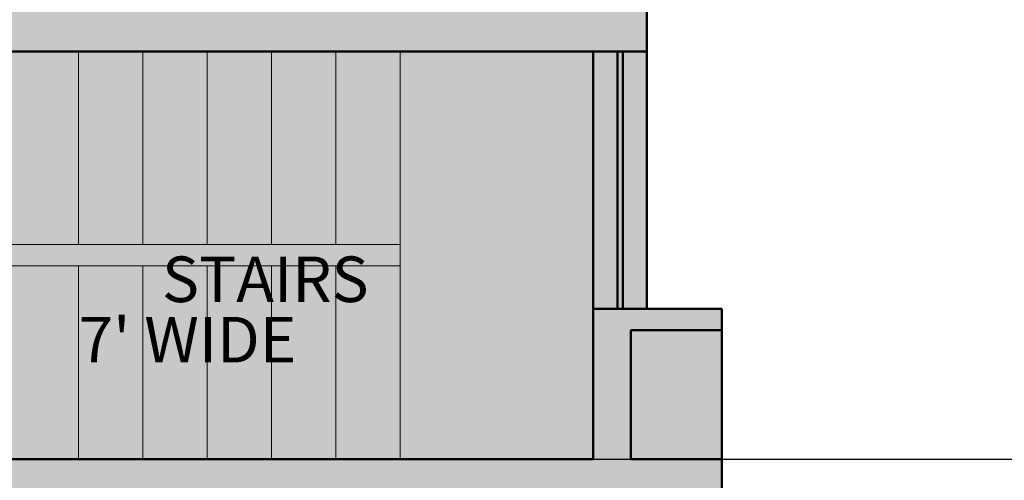
# Model space of a CAD drawing. Units: inches. Extents: x 925 to 2834, y 111 to 1355.
# Tile 8 of 25: x 1602 to 1785, y 638 to 723. Entities that reach past the tile are written whole.
import ezdxf

# ---------------------------------------------------------------- set-up
doc = ezdxf.new("R2010")
doc.units = ezdxf.units.IN
doc.header["$MEASUREMENT"] = 0
for name, color, linetype, lineweight in [('A-ANNO-DIMS', 2, 'Continuous', 18), ('A-AREA-IDEN', 7, 'Continuous', 18), ('A-FLOR-PATT', 252, 'Continuous', 13), ('A-FLOR-STRS', 4, 'Continuous', 18), ('A-WALL', 7, 'Continuous', 50), ('A-WALL-PATT', 8, 'Continuous', 13)]:
    doc.layers.add(name, color=color, linetype=linetype, lineweight=lineweight)
doc.styles.get("Standard").update_dxf_attribs({"font": 'arial.ttf'})
doc.dimstyles.get("Standard").update_dxf_attribs({"dimtxt": 6, "dimasz": 3, "dimexe": 0.18, "dimexo": 0.0625, "dimgap": 0.09, "dimtad": 0, "dimtih": 1, "dimtoh": 1, "dimdec": 1, "dimzin": 0, "dimdsep": 46, "dimlunit": 3, "dimtxsty": 'Standard', "dimblk": 'ARCHTICK', "dimcen": 0.09, "dimadec": 0, "dimazin": 0, "dimtfac": 1, "dimtdec": 1, "dimtofl": 0, "dimtmove": 0, "dimatfit": 3, "dimfxl": 1, "dimtolj": 1, "dimtzin": 0, "dimarcsym": 0})

# ---------------------------------------------------------------- blocks, each defined once
blk = doc.blocks.new('_ArchTick')
at = {"color": 0, "linetype": 'ByBlock', "const_width": 0.15}
blk.add_lwpolyline([(-0.5, -0.5), (0.5, 0.5)], dxfattribs=at)
blk = doc.blocks.new('*D44')
at = {"layer": 'A-ANNO-DIMS', "color": 0, "lineweight": -2, "transparency": 16777216}
for p, q in [((1708.78, 641.59), (1988.62, 641.59)), ((1988.44, 641.59), (1988.44, 516.49)), ((1988.44, 385.09), (1988.44, 510.19)), ((1718.78, 385.09), (1988.62, 385.09))]:
    blk.add_line(p, q, dxfattribs=at)
at = {"layer": 'Defpoints', "color": 0, "transparency": 16777216}
for p in [(1708.71, 641.59), (1988.44, 641.59), (1718.71, 385.09)]:
    blk.add_point(p, dxfattribs=at)
at = {"layer": 'A-ANNO-DIMS', "color": 0, "lineweight": -2, "transparency": 16777216, "xscale": 3, "yscale": 3, "zscale": 3}
for p, rotation in [((1988.44, 641.59), 90), ((1988.44, 385.09), 270)]:
    blk.add_blockref('_ArchTick', p, dxfattribs=dict(at, rotation=rotation))
at = {"layer": 'A-ANNO-DIMS', "color": 0, "transparency": 16777216, "insert": (1988.44, 513.34), "char_height": 6, "attachment_point": 5}
blk.add_mtext('\\A1;256.5', dxfattribs=at)
blk = doc.blocks.new('*D45')
at = {"layer": 'A-ANNO-DIMS', "color": 0, "lineweight": -2, "transparency": 16777216}
for p, q in [((1708.78, 727.59), (1988.62, 727.59)), ((1988.44, 727.59), (1988.44, 687.74)), ((1988.44, 641.59), (1988.44, 681.44)), ((1708.78, 641.59), (1988.62, 641.59))]:
    blk.add_line(p, q, dxfattribs=at)
at = {"layer": 'Defpoints', "color": 0, "transparency": 16777216}
for p in [(1708.71, 727.59), (1988.44, 727.59), (1708.71, 641.59)]:
    blk.add_point(p, dxfattribs=at)
at = {"layer": 'A-ANNO-DIMS', "color": 0, "lineweight": -2, "transparency": 16777216, "xscale": 3, "yscale": 3, "zscale": 3}
for p, rotation in [((1988.44, 727.59), 90), ((1988.44, 641.59), 270)]:
    blk.add_blockref('_ArchTick', p, dxfattribs=dict(at, rotation=rotation))
at = {"layer": 'A-ANNO-DIMS', "color": 0, "transparency": 16777216, "insert": (1988.44, 684.59), "char_height": 6, "attachment_point": 5}
blk.add_mtext('\\A1;86', dxfattribs=at)

msp = doc.modelspace()

# ---------------------------------------------------------------- hatches: boundary and pattern name
at = {"layer": 'A-FLOR-PATT', "transparency": 33554605}
h = msp.add_hatch(color=256, dxfattribs=at)
h.dxf.hatch_style = 1
h.paths.add_polyline_path([(1931.688, 1294.5638), (991.7375, 1294.5638), (991.7375, 172.1134), (1931.688, 172.1134)])
h.paths.add_polyline_path([(1910.7128, 1273.5886), (1910.7128, 193.0886), (1012.7128, 193.0886), (1012.7128, 1273.5886)], flags=16)
h.paths.add_polyline_path([(1850.7128, 1213.5886), (1850.7128, 253.0886), (1072.7128, 253.0886), (1072.7128, 1213.5886)], flags=0)
h.paths.add_polyline_path([(1838.7128, 1201.5886), (1838.7128, 265.0886), (1084.7128, 265.0886), (1084.7128, 530.5886), (1084.7128, 1201.5886)], flags=0)
h.paths.add_polyline_path([(1547.6758, 1155.7396), (1547.6758, 1119.115), (1513.0687, 1119.115), (1513.0687, 1155.7396)], flags=0)
h.paths.add_polyline_path([(1600.1067, 1154.9439), (1634.7139, 1154.9439), (1634.7139, 1119.115), (1600.1067, 1119.115)], flags=0)
h.paths.add_polyline_path([(1505.2502, 1144.5358), (1505.2502, 1119.115), (1470.643, 1119.115), (1470.643, 1144.5358)], flags=0)
h.paths.add_polyline_path([(1559.1357, 1141.0962), (1593.7428, 1141.0962), (1593.7428, 1119.115), (1559.1357, 1119.115)], flags=0)
h.paths.add_polyline_path([(1462.8966, 1154.9439), (1462.8966, 1119.115), (1428.2895, 1119.115), (1428.2895, 1154.9439)], flags=0)
h.paths.add_polyline_path([(1642.4603, 1144.5358), (1677.0675, 1144.5358), (1677.0675, 1119.115), (1642.4603, 1119.115)], flags=0)
h.paths.add_polyline_path([(1422.3508, 1141.0962), (1422.3508, 1119.115), (1387.7436, 1119.115), (1387.7436, 1141.0962)], flags=0)
h.paths.add_polyline_path([(1684.8859, 1155.7396), (1719.4931, 1155.7396), (1719.4931, 1119.115), (1684.8859, 1119.115)], flags=0)
h.paths.add_polyline_path([(1718.7128, 1081.5886), (1718.7128, 1050.1249), (1715.7128, 1050.1249), (1715.7128, 1026.1249), (1715.7128, 1002.1249), (1718.7128, 1002.1249), (1730.7128, 1002.1249), (1730.7128, 998.1249), (1730.7128, 990.1249), (1730.7128, 986.1249), (1718.7128, 986.1249), (1718.7128, 893.5886), (1715.3735, 893.5886), (1715.3735, 891.5886), (1713.3735, 891.5886, 0.41421356), (1677.3735, 855.5886), (1713.3735, 855.5886), (1713.3735, 853.5886), (1715.3735, 853.5886), (1715.3735, 851.5886), (1718.7128, 851.5886), (1718.7128, 821.5865), (1734.4655, 821.5865), (1734.3735, 819.5886, -0.41421356), (1712.4415, 793.5886), (1712.4415, 791.5886), (1718.7128, 791.5886), (1718.7128, 717.5886), (1718.7128, 669.5886), (1732.7128, 669.5886), (1732.7128, 665.5886), (1732.7128, 641.5886), (1732.7128, 634.5886), (1732.7128, 610.5886), (1732.7128, 603.5886), (1718.7128, 603.5886), (1718.7128, 385.0886), (1434.2128, 385.0886), (1434.2128, 530.5886), (1410.2128, 530.5886), (1408.2128, 530.5886), (1408.2128, 532.5886, 0.41421356), (1372.2128, 568.5886), (1372.2128, 532.5886), (1370.2128, 532.5886), (1370.2128, 530.5886), (1368.2128, 530.5886), (1282.2128, 530.5886), (1210.2128, 530.5886), (1200.2128, 530.5886), (1200.2128, 542.1915), (1183.2307, 542.1915), (1183.2307, 546.1915), (1200.2128, 546.1915), (1200.2128, 572.1915), (1183.2307, 572.1915), (1183.2307, 576.1915), (1200.2128, 576.1915), (1200.2128, 727.5886), (1210.2128, 727.5886), (1234.2128, 727.5886), (1259.7128, 727.5886), (1259.7128, 775.5886), (1259.7128, 799.5886), (1259.7128, 847.5886), (1259.7128, 993.5872), (1259.7128, 1065.5872), (1259.7128, 1071.5886), (1219.6318, 1071.5886), (1219.6318, 1081.5886), (1084.7128, 1081.5886), (1084.7128, 1119.115), (1256.8974, 1119.115), (1256.8974, 1154.9439), (1291.5046, 1154.9439), (1291.5046, 1119.115), (1256.8974, 1119.115), (1256.6723, 1081.5886), (1293.7128, 1081.5886), (1341.7128, 1081.5886), (1341.7128, 1093.5886), (1347.7128, 1093.5886), (1371.7128, 1093.5886), (1377.7128, 1093.5886), (1377.7128, 1081.5886), (1668.7128, 1081.5886), (1668.7128, 1117.5886), (1675.7128, 1117.5886), (1711.7128, 1117.5886), (1718.7128, 1117.5886)], flags=0)
h.paths.add_polyline_path([(1376.2838, 1155.7396), (1376.2838, 1119.115), (1341.6766, 1119.115), (1341.6766, 1155.7396)], flags=0)
h.paths.add_polyline_path([(1341.7128, 1076.0886), (1293.7128, 1076.0886), (1293.7128, 1071.5886), (1269.7128, 1071.5886), (1269.7128, 1065.5872), (1266.7128, 1065.5872), (1266.7128, 1029.5872), (1265.7128, 1029.5872), (1265.7128, 993.5872), (1269.7128, 993.5872), (1269.7128, 903.5886), (1269.7128, 893.5886), (1269.7128, 847.5886), (1265.2128, 847.5886), (1265.2128, 799.5886), (1269.7128, 799.5886), (1269.7128, 775.5886), (1265.2128, 775.5886), (1265.2128, 727.5886), (1269.7128, 727.5886), (1444.2128, 727.5886), (1444.2128, 717.5886), (1234.2128, 717.5886), (1234.2128, 722.0886), (1210.2128, 722.0886), (1210.2128, 717.5886), (1210.2128, 540.5886), (1210.2128, 536.0886), (1282.2128, 536.0886), (1282.2128, 535.0886), (1210.2128, 535.0886), (1210.2128, 540.5886), (1210.2128, 717.5886), (1210.2128, 723.0886), (1234.2128, 723.0886), (1234.2128, 717.5886), (1444.2128, 717.5886), (1444.2128, 727.5886), (1269.7128, 727.5886), (1264.2128, 727.5886), (1264.2128, 775.5886), (1269.7128, 775.5886), (1269.7128, 799.5886), (1264.2128, 799.5886), (1264.2128, 847.5886), (1269.7128, 847.5886), (1269.7128, 893.5886), (1269.7128, 903.5886), (1269.7128, 993.5872), (1264.7128, 993.5872), (1264.7128, 1029.5872), (1265.7128, 1029.5872), (1265.7128, 1065.5872), (1269.7128, 1065.5872), (1269.7128, 1071.5886), (1293.7128, 1071.5886), (1293.7128, 1077.0886), (1341.7128, 1077.0886)], flags=0)
h.paths.add_polyline_path([(1730.9529, 1141.0962), (1765.5601, 1141.0962), (1765.5601, 1119.115), (1730.9529, 1119.115)], flags=0)
h.paths.add_polyline_path([(1333.8582, 1144.5358), (1333.8582, 1119.115), (1299.251, 1119.115), (1299.251, 1144.5358)], flags=0)
h.paths.add_polyline_path([(1592.7128, 968.5886), (1596.0342, 968.5886), (1602.7128, 968.5886), (1708.7128, 968.5886), (1708.7128, 903.5886), (1602.7128, 903.5886), (1602.7128, 938.5886), (1592.7128, 938.5886), (1592.7128, 903.5886), (1451.7128, 903.5886), (1451.7128, 893.5886), (1511.7128, 893.5886), (1511.7128, 881.5886), (1515.2128, 881.5886), (1518.7128, 881.5886), (1518.7128, 893.5886), (1592.7128, 893.5886), (1592.7128, 799.5886), (1518.7128, 799.5886), (1518.7128, 857.5886), (1511.7128, 857.5886), (1511.7128, 799.5886), (1511.7128, 772.0886), (1521.7128, 772.0886), (1521.7128, 792.5886), (1592.7128, 792.5886), (1592.7128, 727.5886), (1521.7128, 727.5886), (1521.7128, 748.0886), (1511.7128, 748.0886), (1511.7128, 717.5886), (1708.7128, 717.5886), (1714.2128, 717.5886), (1714.2128, 669.5886), (1708.7128, 669.5886), (1708.7128, 641.5886), (1492.2128, 641.5886), (1492.2128, 631.5886), (1621.2128, 631.5886), (1621.2128, 443.0886), (1625.7128, 443.0886), (1625.7128, 503.0886), (1625.7128, 507.5886), (1625.7128, 631.5886), (1708.7128, 631.5886), (1708.7128, 507.5886), (1655.7128, 507.5886), (1655.7128, 503.0886), (1708.7128, 503.0886), (1708.7128, 395.0886), (1625.7128, 395.0886), (1625.7128, 419.0886), (1621.2128, 419.0886), (1621.2128, 395.0886), (1482.2128, 395.0886), (1482.2128, 385.0886), (1434.2128, 385.0886), (1434.2128, 433.0886), (1444.2128, 433.0886), (1444.2128, 631.5886), (1450.2128, 631.5886), (1450.2128, 634.91), (1452.2128, 634.91), (1452.2128, 669.5886), (1454.2128, 669.5886, -0.40021217), (1490.1712, 635.3173), (1492.2128, 635.3173), (1492.2128, 641.5886), (1564.7128, 641.5886), (1564.7128, 677.5886), (1672.7128, 677.5886), (1672.7128, 681.5886), (1564.7128, 681.5886), (1564.7128, 717.5886), (1511.7128, 717.5886), (1511.7128, 748.0886), (1511.7128, 772.0886), (1511.7128, 799.5886), (1511.7128, 857.5886), (1511.8913, 857.5886), (1511.8913, 859.5886), (1515.6201, 859.5886, 0.41421356), (1537.552, 879.5886), (1513.552, 879.5886), (1511.8913, 879.5886), (1511.8913, 881.5886), (1511.7128, 881.5886), (1511.7128, 893.5886), (1451.7128, 893.5886), (1451.7128, 903.5886), (1592.7128, 903.5886), (1592.7128, 938.5886), (1592.7128, 940.5886), (1596.4415, 940.5886, 0.41421356), (1618.3735, 966.5886), (1594.3735, 966.5886), (1592.7128, 966.5886)], flags=0)
h.paths.add_polyline_path([(1377.7128, 903.5886), (1377.7128, 893.5886), (1305.7128, 893.5886), (1305.7128, 903.5886)], flags=0)
h.paths.add_polyline_path([(1708.7128, 821.5886), (1712.0342, 821.5886), (1712.0342, 819.5886), (1710.3735, 819.5886), (1708.7128, 819.5886)], flags=0)
h.paths.add_polyline_path([(1576.7128, 695.1992), (1575.5896, 693.6649), (1575.9687, 694.6994), (1575.4438, 695.1992), (1575.9687, 695.699), (1575.5896, 696.7335)], flags=0)
h.paths.add_polyline_path([(1565.9817, 662.3134), (1565.4568, 661.8136), (1565.8359, 660.7791), (1564.7128, 662.3134), (1565.8359, 663.8477), (1565.4568, 662.8132)], flags=0)
h.paths.add_polyline_path([(1444.2128, 433.0886), (1444.2128, 395.0886), (1482.2128, 395.0886), (1482.2128, 389.0886), (1438.2128, 389.0886), (1438.2128, 391.8608), (1438.2128, 433.0886)], flags=0)
h.paths.add_polyline_path([(1410.2128, 506.5886), (1410.2128, 289.0886), (1108.7128, 289.0886), (1108.7128, 506.5886)], flags=0)
h.paths.add_polyline_path([(1612.3153, 838.3016), (1680.4151, 838.3016), (1680.4151, 851.3131), (1612.3153, 851.3131)], flags=8)
h.paths.add_polyline_path([(1208.3174, 395.0436), (1282.1017, 395.0436), (1282.1017, 408.0552), (1208.3174, 408.0552)], flags=8)
h.paths.add_polyline_path([(1291.8049, 598.7427), (1369.8017, 598.7427), (1369.8017, 611.7542), (1291.8049, 611.7542)], flags=8)
h.paths.add_polyline_path([(1119.679, 917.3022), (1191.0817, 917.3022), (1191.0817, 930.3137), (1119.679, 930.3137)], flags=8)
h.paths.add_polyline_path([(1332.2261, 815.9808), (1410.2258, 815.9808), (1410.2258, 829.001), (1332.2261, 829.001)], flags=8)
h.paths.add_polyline_path([(1390.9013, 955.8158), (1475.4981, 955.8158), (1475.4981, 968.8273), (1390.9013, 968.8273)], flags=8)
h.paths.add_polyline_path([(1620.3436, 998.9325), (1688.4434, 998.9325), (1688.4434, 1011.944), (1620.3436, 1011.944)], flags=8)
h.paths.add_polyline_path([(1620.3436, 914.1039), (1691.7405, 914.1039), (1691.7405, 927.1155), (1620.3436, 927.1155)], flags=8)
h.paths.add_polyline_path([(1521.4542, 816.005), (1589.5569, 816.005), (1589.5569, 829.0253), (1521.4542, 829.0253)], flags=8)
h.paths.add_polyline_path([(1528.524, 740.3497), (1602.3082, 740.3497), (1602.3082, 753.3613), (1528.524, 753.3613)], flags=8)
h.paths.add_polyline_path([(1627.6094, 762.6128), (1702.3091, 762.6128), (1702.3091, 775.6244), (1627.6094, 775.6244)], flags=8)
h.paths.add_polyline_path([(1610.5442, 657.2751), (1684.3284, 657.2751), (1684.3284, 670.2867), (1610.5442, 670.2867)], flags=8)
h.paths.add_polyline_path([(1636.6983, 519.472), (1711.3981, 519.472), (1711.3981, 532.4835), (1636.6983, 532.4835)], flags=8)
h.paths.add_polyline_path([(1616.8577, 424.8539), (1694.8545, 424.8539), (1694.8545, 437.8654), (1616.8577, 437.8654)], flags=8)
h.paths.add_polyline_path([(1506.1456, 460.8838), (1579.9299, 460.8838), (1579.9299, 473.8953), (1506.1456, 473.8953)], flags=8)
h.paths.add_polyline_path([(1624.6119, 784.6011), (1696.9185, 784.6011), (1696.9185, 797.7864), (1624.6119, 797.7864)], flags=8)
h.paths.add_polyline_path([(1606.3732, 854.2194), (1683.3039, 854.2194), (1683.3039, 867.4048), (1606.3732, 867.4048)], flags=8)
h.paths.add_polyline_path([(1127.8008, 940.3581), (1165.1637, 940.3581), (1165.1637, 953.5348), (1127.8008, 953.5348)], flags=8)
h.paths.add_polyline_path([(1620.8657, 1019.4968), (1677.3447, 1019.4968), (1677.3447, 1032.6735), (1620.8657, 1032.6735)], flags=8)
h.paths.add_polyline_path([(1620.8643, 930.1821), (1703.0564, 930.1821), (1703.0564, 943.3675), (1620.8643, 943.3675)], flags=8)
h.paths.add_polyline_path([(1324.5702, 836.8338), (1408.0892, 836.8338), (1408.0892, 850.0191), (1324.5702, 850.0191)], flags=8)
h.paths.add_polyline_path([(1281.6584, 622.8885), (1383.6213, 622.8885), (1383.6213, 636.0739), (1281.6584, 636.0739)], flags=8)
h.paths.add_polyline_path([(1210.6721, 416.7893), (1269.1299, 416.7893), (1269.1299, 429.9747), (1210.6721, 429.9747)], flags=8)
h.paths.add_polyline_path([(1507.8264, 477.4836), (1586.7329, 477.4836), (1586.7329, 490.669), (1507.8264, 490.669)], flags=8)
h.paths.add_polyline_path([(1643.6238, 443.8135), (1696.6696, 443.8135), (1696.6696, 456.5643), (1643.6238, 456.5643)], flags=8)
h.paths.add_polyline_path([(1647.2466, 540.5638), (1693.1825, 540.5638), (1693.1825, 553.7491), (1647.2466, 553.7491)], flags=8)
h.paths.add_polyline_path([(1626.0633, 668.5064), (1673.3174, 668.5064), (1673.3174, 681.6831), (1626.0633, 681.6831)], flags=8)
h.paths.add_polyline_path([(1538.2915, 830.7872), (1567.5942, 830.7872), (1567.5942, 843.5293), (1538.2915, 843.5293)], flags=8)
h.paths.add_polyline_path([(1530.9338, 754.0477), (1559.576, 754.0477), (1559.576, 766.7898), (1530.9338, 766.7898)], flags=8)
h.paths.add_polyline_path([(1351.2461, 979.2309), (1513.8919, 979.2309), (1513.8919, 992.4076), (1351.2461, 992.4076)], flags=8)
at = {"layer": 'A-FLOR-PATT'}
h = msp.add_hatch(color=256, dxfattribs=at)
h.dxf.hatch_style = 1
h.paths.add_polyline_path([(1850.7128, 1213.5886), (1072.7128, 1213.5886), (1072.7128, 253.0886), (1850.7128, 253.0886)])
h.paths.add_polyline_path([(1084.7128, 1201.5886), (1838.7128, 1201.5886), (1838.7128, 265.0886), (1084.7128, 265.0886)], flags=16)
h.paths.add_polyline_path([(1183.2307, 576.1915), (1200.2128, 576.1915), (1200.2128, 727.5886), (1210.2128, 727.5886), (1234.2128, 727.5886), (1259.7128, 727.5886), (1259.7128, 775.5886), (1259.7128, 799.5886), (1259.7128, 847.5886), (1259.7128, 993.5872), (1259.7128, 1065.5872), (1259.7128, 1071.5886), (1219.6318, 1071.5886), (1219.6318, 1081.5886), (1293.7128, 1081.5886), (1341.7128, 1081.5886), (1341.7128, 1093.5886), (1347.7128, 1093.5886), (1347.7128, 1081.5886), (1371.7128, 1081.5886), (1371.7128, 1093.5886), (1377.7128, 1093.5886), (1377.7128, 1081.5886), (1668.7128, 1081.5886), (1668.7128, 1117.5886), (1675.7128, 1117.5886), (1675.7128, 1081.5886), (1711.7128, 1081.5886), (1711.7128, 1117.5886), (1718.7128, 1117.5886), (1718.7128, 1081.5886), (1718.7128, 1050.1249), (1715.7128, 1050.1249), (1715.7128, 1026.1249), (1715.7128, 1002.1249), (1718.7128, 1002.1249), (1730.7128, 1002.1249), (1730.7128, 998.1249), (1730.7128, 990.1249), (1730.7128, 986.1249), (1718.7128, 986.1249), (1718.7128, 893.5886), (1715.3735, 893.5886), (1715.3735, 891.5886), (1713.3735, 891.5886, 0.41421356), (1677.3735, 855.5886), (1713.3735, 855.5886), (1713.3735, 853.5886), (1715.3735, 853.5886), (1715.3735, 851.5886), (1718.7128, 851.5886), (1718.7128, 821.5865), (1734.4655, 821.5865), (1734.3735, 819.5886, -0.41421356), (1712.4415, 793.5886), (1712.4415, 791.5886), (1718.7128, 791.5886), (1718.7128, 717.5886), (1718.7128, 669.5886), (1732.7128, 669.5886), (1732.7128, 665.5886), (1732.7128, 641.5886), (1732.7128, 634.5886), (1732.7128, 610.5886), (1732.7128, 603.5886), (1718.7128, 603.5886), (1718.7128, 385.0886), (1434.2128, 385.0886), (1434.2128, 433.0886), (1434.2128, 530.5886), (1410.2128, 530.5886), (1408.2128, 530.5886), (1408.2128, 532.5886, 0.41421356), (1372.2128, 568.5886), (1372.2128, 532.5886), (1370.2128, 532.5886), (1370.2128, 530.5886), (1368.2128, 530.5886), (1282.2128, 530.5886), (1210.2128, 530.5886), (1200.2128, 530.5886), (1200.2128, 542.1915), (1183.2307, 542.1915), (1183.2307, 546.1915), (1200.2128, 546.1915), (1200.2128, 572.1915), (1183.2307, 572.1915)], flags=0)
h.paths.add_polyline_path([(1210.2128, 717.5886), (1210.2128, 723.0886), (1234.2128, 723.0886), (1234.2128, 717.5886), (1444.2128, 717.5886), (1444.2128, 727.5886), (1269.7128, 727.5886), (1264.2128, 727.5886), (1264.2128, 775.5886), (1269.7128, 775.5886), (1269.7128, 799.5886), (1264.2128, 799.5886), (1264.2128, 847.5886), (1269.7128, 847.5886), (1269.7128, 893.5886), (1269.7128, 903.5886), (1269.7128, 993.5872), (1264.7128, 993.5872), (1264.7128, 1029.5872), (1265.7128, 1029.5872), (1265.7128, 1065.5872), (1269.7128, 1065.5872), (1269.7128, 1071.5886), (1293.7128, 1071.5886), (1293.7128, 1077.0886), (1341.7128, 1077.0886), (1341.7128, 1076.0886), (1293.7128, 1076.0886), (1293.7128, 1071.5886), (1269.7128, 1071.5886), (1269.7128, 1065.5872), (1266.7128, 1065.5872), (1266.7128, 1029.5872), (1265.7128, 1029.5872), (1265.7128, 993.5872), (1269.7128, 993.5872), (1269.7128, 903.5886), (1269.7128, 893.5886), (1269.7128, 847.5886), (1265.2128, 847.5886), (1265.2128, 799.5886), (1269.7128, 799.5886), (1269.7128, 775.5886), (1265.2128, 775.5886), (1265.2128, 727.5886), (1269.7128, 727.5886), (1444.2128, 727.5886), (1444.2128, 717.5886), (1234.2128, 717.5886), (1234.2128, 722.0886), (1210.2128, 722.0886), (1210.2128, 717.5886), (1210.2128, 540.5886), (1210.2128, 536.0886), (1282.2128, 536.0886), (1282.2128, 535.0886), (1210.2128, 535.0886), (1210.2128, 540.5886)], flags=0)
h.paths.add_polyline_path([(1450.2128, 634.91), (1452.2128, 634.91), (1452.2128, 669.5886), (1454.2128, 669.5886, -0.40021217), (1490.1712, 635.3173), (1492.2128, 635.3173), (1492.2128, 641.5886), (1564.7128, 641.5886), (1564.7128, 677.5886), (1672.7128, 677.5886), (1672.7128, 681.5886), (1564.7128, 681.5886), (1564.7128, 717.5886), (1511.7128, 717.5886), (1511.7128, 748.0886), (1511.7128, 772.0886), (1511.7128, 799.5886), (1511.7128, 857.5886), (1511.8913, 857.5886), (1511.8913, 859.5886), (1515.6201, 859.5886, 0.41421356), (1537.552, 879.5886), (1513.552, 879.5886), (1511.8913, 879.5886), (1511.8913, 881.5886), (1511.7128, 881.5886), (1511.7128, 893.5886), (1451.7128, 893.5886), (1451.7128, 903.5886), (1592.7128, 903.5886), (1592.7128, 938.5886), (1592.7128, 940.5886), (1596.4415, 940.5886, 0.41421356), (1618.3735, 966.5886), (1594.3735, 966.5886), (1592.7128, 966.5886), (1592.7128, 968.5886), (1596.0342, 968.5886), (1602.7128, 968.5886), (1708.7128, 968.5886), (1708.7128, 903.5886), (1602.7128, 903.5886), (1602.7128, 938.5886), (1592.7128, 938.5886), (1592.7128, 903.5886), (1451.7128, 903.5886), (1451.7128, 893.5886), (1511.7128, 893.5886), (1511.7128, 881.5886), (1518.7128, 881.5886), (1518.7128, 893.5886), (1592.7128, 893.5886), (1592.7128, 799.5886), (1518.7128, 799.5886), (1518.7128, 857.5886), (1511.7128, 857.5886), (1511.7128, 799.5886), (1511.7128, 772.0886), (1521.7128, 772.0886), (1521.7128, 792.5886), (1592.7128, 792.5886), (1592.7128, 727.5886), (1521.7128, 727.5886), (1521.7128, 748.0886), (1511.7128, 748.0886), (1511.7128, 717.5886), (1708.7128, 717.5886), (1714.2128, 717.5886), (1714.2128, 669.5886), (1708.7128, 669.5886), (1708.7128, 641.5886), (1492.2128, 641.5886), (1492.2128, 631.5886), (1621.2128, 631.5886), (1621.2128, 443.0886), (1625.7128, 443.0886), (1625.7128, 503.0886), (1625.7128, 507.5886), (1625.7128, 631.5886), (1708.7128, 631.5886), (1708.7128, 507.5886), (1655.7128, 507.5886), (1655.7128, 503.0886), (1708.7128, 503.0886), (1708.7128, 395.0886), (1625.7128, 395.0886), (1625.7128, 419.0886), (1621.2128, 419.0886), (1621.2128, 395.0886), (1482.2128, 395.0886), (1482.2128, 389.0886), (1438.2128, 389.0886), (1438.2128, 391.8608), (1438.2128, 433.0886), (1444.2128, 433.0886), (1444.2128, 631.5886), (1450.2128, 631.5886)], flags=0)
h.paths.add_polyline_path([(1444.2128, 433.0886), (1444.2128, 395.0886), (1482.2128, 395.0886), (1482.2128, 391.0886), (1440.2128, 391.0886), (1440.2128, 391.8608), (1440.2128, 433.0886)], flags=0)
h.paths.add_polyline_path([(1305.7128, 893.5886), (1305.7128, 903.5886), (1377.7128, 903.5886), (1377.7128, 893.5886)], flags=0)
h.paths.add_polyline_path([(1564.7128, 662.3134), (1565.8359, 663.8477), (1565.4568, 662.8132), (1565.9817, 662.3134), (1565.4568, 661.8136), (1565.8359, 660.7791)], flags=0)
h.paths.add_polyline_path([(1575.4438, 695.1992), (1575.9687, 695.699), (1575.5896, 696.7335), (1576.7128, 695.1992), (1575.5896, 693.6649), (1575.9687, 694.6994)], flags=0)
h.paths.add_polyline_path([(1708.7128, 821.5886), (1712.0342, 821.5886), (1712.0342, 819.5886), (1710.3735, 819.5886), (1708.7128, 819.5886)], flags=0)
h = msp.add_hatch(color=256, dxfattribs=at)
h.dxf.hatch_style = 1
h.paths.add_polyline_path([(1718.7128, 603.5886), (1708.7128, 603.5886), (1708.7128, 507.5886), (1655.7128, 507.5886), (1655.7128, 503.0886), (1708.7128, 503.0886), (1708.7128, 395.0886), (1625.7128, 395.0886), (1625.7128, 419.0886), (1621.2128, 419.0886), (1621.2128, 395.0886), (1482.2128, 395.0886), (1482.2128, 385.0886), (1718.7128, 385.0886)])
h.paths.add_polyline_path([(1625.7128, 631.5886), (1708.7128, 631.5886), (1708.7128, 603.5886), (1718.7128, 603.5886), (1732.7128, 603.5886), (1732.7128, 610.5886), (1715.7128, 610.5886), (1715.7128, 634.5886), (1732.7128, 634.5886), (1732.7128, 641.5886), (1715.7128, 641.5886), (1715.7128, 665.5886), (1732.7128, 665.5886), (1732.7128, 669.5886), (1708.7128, 669.5886), (1708.7128, 641.5886), (1492.2128, 641.5886), (1492.2128, 631.5886), (1621.2128, 631.5886), (1621.2128, 443.0886), (1625.7128, 443.0886), (1625.7128, 503.0886), (1625.7128, 507.5886)])
h.paths.add_polyline_path([(1718.7128, 851.5886), (1708.7128, 851.5886), (1708.7128, 828.5886), (1602.7128, 828.5886), (1602.7128, 893.5886), (1708.7128, 893.5886), (1718.7128, 893.5886), (1718.7128, 986.1249), (1730.7128, 986.1249), (1730.7128, 990.1249), (1718.7128, 990.1249), (1718.7128, 998.1249), (1730.7128, 998.1249), (1730.7128, 1002.1249), (1718.7128, 1002.1249), (1708.7128, 1002.1249), (1708.7128, 975.5886), (1602.7128, 975.5886), (1602.7128, 1011.5886), (1592.7128, 1011.5886), (1592.7128, 968.5886), (1596.0342, 968.5886), (1602.7128, 968.5886), (1708.7128, 968.5886), (1708.7128, 903.5886), (1602.7128, 903.5886), (1602.7128, 938.5886), (1592.7128, 938.5886), (1592.7128, 903.5886), (1451.7128, 903.5886), (1451.7128, 893.5886), (1511.7128, 893.5886), (1511.7128, 881.5886), (1515.2128, 881.5886), (1518.7128, 881.5886), (1518.7128, 893.5886), (1592.7128, 893.5886), (1592.7128, 799.5886), (1518.7128, 799.5886), (1518.7128, 857.5886), (1511.7128, 857.5886), (1511.7128, 799.5886), (1511.7128, 772.0886), (1521.7128, 772.0886), (1521.7128, 792.5886), (1592.7128, 792.5886), (1592.7128, 727.5886), (1521.7128, 727.5886), (1521.7128, 748.0886), (1511.7128, 748.0886), (1511.7128, 717.5886), (1708.7128, 717.5886), (1718.7128, 717.5886), (1718.7128, 727.5886), (1718.7128, 791.5886), (1708.7128, 791.5886), (1708.7128, 727.5886), (1602.7128, 727.5886), (1602.7128, 821.5886), (1708.7128, 821.5886), (1712.0342, 821.5886), (1718.7128, 821.5886)])
h.paths.add_polyline_path([(1718.7128, 1081.5886), (1718.7128, 1117.5886), (1711.7128, 1117.5886), (1711.7128, 1081.5886), (1675.7128, 1081.5886), (1675.7128, 1117.5886), (1668.7128, 1117.5886), (1668.7128, 1081.5886), (1377.7128, 1081.5886), (1377.7128, 1093.5886), (1371.7128, 1093.5886), (1371.7128, 1081.5886), (1347.7128, 1081.5886), (1347.7128, 1093.5886), (1341.7128, 1093.5886), (1341.7128, 1081.5886), (1341.7128, 1071.5886), (1592.7128, 1071.5886), (1592.7128, 1035.5886), (1602.7128, 1035.5886), (1602.7128, 1071.5886), (1708.7128, 1071.5886), (1708.7128, 1050.1249), (1718.7128, 1050.1249)])
h.paths.add_polyline_path([(1293.7128, 1081.5886), (1219.6318, 1081.5886), (1219.6318, 1071.5886), (1259.7128, 1071.5886), (1259.7128, 1065.5872), (1269.7128, 1065.5872), (1269.7128, 1071.5886), (1293.7128, 1071.5886)])
h.paths.add_polyline_path([(1269.7128, 903.5886), (1269.7128, 993.5872), (1259.7128, 993.5872), (1259.7128, 847.5886), (1269.7128, 847.5886), (1269.7128, 893.5886)])
h.paths.add_polyline_path([(1377.7128, 903.5886), (1305.7128, 903.5886), (1305.7128, 893.5886), (1377.7128, 893.5886)])
h.paths.add_polyline_path([(1444.2128, 727.5886), (1269.7128, 727.5886), (1259.7128, 727.5886), (1234.2128, 727.5886), (1234.2128, 717.5886), (1444.2128, 717.5886)])
h.paths.add_polyline_path([(1269.7128, 799.5886), (1259.7128, 799.5886), (1259.7128, 775.5886), (1269.7128, 775.5886)])
h.paths.add_polyline_path([(1444.2128, 631.5886), (1450.2128, 631.5886), (1450.2128, 634.91), (1450.2128, 641.5886), (1434.2128, 641.5886), (1434.2128, 540.5886), (1410.2128, 540.5886), (1410.2128, 530.5886), (1434.2128, 530.5886), (1434.2128, 433.0886), (1444.2128, 433.0886)])
h.paths.add_polyline_path([(1368.2128, 533.91), (1368.2128, 540.5886), (1282.2128, 540.5886), (1282.2128, 530.5886), (1368.2128, 530.5886)])
h.paths.add_polyline_path([(1210.2128, 717.5886), (1210.2128, 727.5886), (1200.2128, 727.5886), (1200.2128, 576.1915), (1183.2307, 576.1915), (1183.2307, 572.1915), (1200.2128, 572.1915), (1200.2128, 546.1915), (1183.2307, 546.1915), (1183.2307, 542.1915), (1200.2128, 542.1915), (1200.2128, 530.5886), (1210.2128, 530.5886), (1210.2128, 540.5886)])
at = {"layer": 'A-FLOR-PATT', "transparency": 33554605}
h = msp.add_hatch(color=256, dxfattribs=at)
h.dxf.hatch_style = 1
h.paths.add_polyline_path([(1592.7128, 938.5886), (1592.7128, 940.5886), (1596.4415, 940.5886, 0.41421356), (1618.3735, 966.5886), (1594.3735, 966.5886), (1592.7128, 966.5886), (1592.7128, 968.5886), (1592.7128, 1011.5886), (1602.7128, 1011.5886), (1602.7128, 975.5886), (1708.7128, 975.5886), (1708.7128, 1002.1249), (1711.7128, 1002.1249), (1711.7128, 1026.1249), (1711.7128, 1050.1249), (1708.7128, 1050.1249), (1708.7128, 1071.5886), (1602.7128, 1071.5886), (1602.7128, 1035.5886), (1592.7128, 1035.5886), (1592.7128, 1071.5886), (1341.7128, 1071.5886), (1293.7128, 1071.5886), (1269.7128, 1071.5886), (1269.7128, 1065.5872), (1269.7128, 993.5872), (1269.7128, 903.5886), (1269.7128, 893.5886), (1269.7128, 847.5886), (1269.7128, 799.5886), (1269.7128, 775.5886), (1269.7128, 727.5886), (1444.2128, 727.5886), (1444.2128, 717.5886), (1234.2128, 717.5886), (1210.2128, 717.5886), (1210.2128, 540.5886), (1282.2128, 540.5886), (1368.2128, 540.5886), (1368.2128, 533.91), (1370.2128, 533.91), (1370.2128, 568.5886), (1372.2128, 568.5886, -0.40021217), (1408.1712, 534.3173), (1410.2128, 534.3173), (1410.2128, 540.5886), (1434.2128, 540.5886), (1434.2128, 641.5886), (1450.2128, 641.5886), (1450.2128, 634.91), (1452.2128, 634.91), (1452.2128, 669.5886), (1454.2128, 669.5886, -0.40021217), (1490.1712, 635.3173), (1492.2128, 635.3173), (1492.2128, 641.5886), (1564.7128, 641.5886), (1564.7128, 677.5886), (1672.7128, 677.5886), (1672.7128, 681.5886), (1564.7128, 681.5886), (1564.7128, 717.5886), (1511.7128, 717.5886), (1511.7128, 748.0886), (1511.7128, 772.0886), (1511.7128, 799.5886), (1511.7128, 857.5886), (1511.8913, 857.5886), (1511.8913, 859.5886), (1515.6201, 859.5886, 0.41421356), (1537.552, 879.5886), (1513.552, 879.5886), (1511.8913, 879.5886), (1511.8913, 881.5886), (1511.7128, 881.5886), (1511.7128, 893.5886), (1451.7128, 893.5886), (1451.7128, 903.5886), (1592.7128, 903.5886)])
h.paths.add_polyline_path([(1377.7128, 903.5886), (1377.7128, 893.5886), (1305.7128, 893.5886), (1305.7128, 903.5886)], flags=16)
h.paths.add_polyline_path([(1592.7128, 893.5886), (1518.7128, 893.5886), (1518.7128, 881.5865), (1537.6441, 881.5865), (1537.552, 879.5886, -0.41421356), (1515.6201, 859.5886), (1515.6201, 857.5886), (1518.7128, 857.5886), (1518.7128, 799.5886), (1592.7128, 799.5886)], flags=17)
h.paths.add_polyline_path([(1291.8049, 598.7427), (1369.8017, 598.7427), (1369.8017, 611.7542), (1291.8049, 611.7542)], flags=24)
h.paths.add_polyline_path([(1332.2261, 815.9808), (1410.2258, 815.9808), (1410.2258, 829.001), (1332.2261, 829.001)], flags=24)
h.paths.add_polyline_path([(1390.9013, 955.8158), (1475.4981, 955.8158), (1475.4981, 968.8273), (1390.9013, 968.8273)], flags=24)
h.paths.add_polyline_path([(1620.3436, 998.9325), (1688.4434, 998.9325), (1688.4434, 1011.944), (1620.3436, 1011.944)], flags=24)
h.paths.add_polyline_path([(1620.8657, 1019.4968), (1677.3447, 1019.4968), (1677.3447, 1032.6735), (1620.8657, 1032.6735)], flags=24)
h.paths.add_polyline_path([(1324.5702, 836.8338), (1408.0892, 836.8338), (1408.0892, 850.0191), (1324.5702, 850.0191)], flags=24)
h.paths.add_polyline_path([(1281.6584, 622.8885), (1383.6213, 622.8885), (1383.6213, 636.0739), (1281.6584, 636.0739)], flags=24)
h.paths.add_polyline_path([(1626.0633, 668.5064), (1673.3174, 668.5064), (1673.3174, 681.6831), (1626.0633, 681.6831)], flags=25)
h.paths.add_polyline_path([(1351.2461, 979.2309), (1513.8919, 979.2309), (1513.8919, 992.4076), (1351.2461, 992.4076)], flags=24)
h.paths.add_polyline_path([(1521.4542, 816.005), (1589.5569, 816.005), (1589.5569, 829.0253), (1521.4542, 829.0253)], flags=24)
h.paths.add_polyline_path([(1538.2915, 830.7872), (1567.5942, 830.7872), (1567.5942, 843.5293), (1538.2915, 843.5293)], flags=24)
h.paths.add_polyline_path([(1636.6983, 519.472), (1711.3981, 519.472), (1711.3981, 532.4835), (1636.6983, 532.4835)], flags=9)
h.paths.add_polyline_path([(1616.8577, 424.8539), (1694.8545, 424.8539), (1694.8545, 437.8654), (1616.8577, 437.8654)], flags=9)
h.paths.add_polyline_path([(1506.1456, 460.8838), (1579.9299, 460.8838), (1579.9299, 473.8953), (1506.1456, 473.8953)], flags=9)
h.paths.add_polyline_path([(1606.3732, 854.2194), (1683.3039, 854.2194), (1683.3039, 867.4048), (1606.3732, 867.4048)], flags=25)
h.paths.add_polyline_path([(1507.8264, 477.4836), (1586.7329, 477.4836), (1586.7329, 490.669), (1507.8264, 490.669)], flags=9)
h.paths.add_polyline_path([(1643.6238, 443.8135), (1696.6696, 443.8135), (1696.6696, 456.5643), (1643.6238, 456.5643)], flags=9)
h.paths.add_polyline_path([(1647.2466, 540.5638), (1693.1825, 540.5638), (1693.1825, 553.7491), (1647.2466, 553.7491)], flags=25)
h = msp.add_hatch(color=256, dxfattribs=at)
h.dxf.hatch_style = 1
h.paths.add_polyline_path([(1200.2128, 727.5886), (1084.7128, 727.5886), (1084.7128, 530.5886), (1200.2128, 530.5886), (1200.2128, 542.1915), (1183.2307, 542.1915), (1183.2307, 546.1915), (1200.2128, 546.1915), (1200.2128, 572.1915), (1183.2307, 572.1915), (1183.2307, 576.1915), (1200.2128, 576.1915)])
h.paths.add_polyline_path([(1612.3153, 838.3016), (1680.4151, 838.3016), (1680.4151, 851.3131), (1612.3153, 851.3131)], flags=9)
h.paths.add_polyline_path([(1291.8049, 598.7427), (1369.8017, 598.7427), (1369.8017, 611.7542), (1291.8049, 611.7542)], flags=9)
h.paths.add_polyline_path([(1119.679, 917.3022), (1191.0817, 917.3022), (1191.0817, 930.3137), (1119.679, 930.3137)], flags=9)
h.paths.add_polyline_path([(1332.2261, 815.9808), (1410.2258, 815.9808), (1410.2258, 829.001), (1332.2261, 829.001)], flags=9)
h.paths.add_polyline_path([(1390.9013, 955.8158), (1475.4981, 955.8158), (1475.4981, 968.8273), (1390.9013, 968.8273)], flags=9)
h.paths.add_polyline_path([(1620.3436, 998.9325), (1688.4434, 998.9325), (1688.4434, 1011.944), (1620.3436, 1011.944)], flags=9)
h.paths.add_polyline_path([(1620.3436, 914.1039), (1691.7405, 914.1039), (1691.7405, 927.1155), (1620.3436, 927.1155)], flags=9)
h.paths.add_polyline_path([(1521.4542, 816.005), (1589.5569, 816.005), (1589.5569, 829.0253), (1521.4542, 829.0253)], flags=9)
h.paths.add_polyline_path([(1522.4337, 740.3497), (1596.218, 740.3497), (1596.218, 753.3613), (1522.4337, 753.3613)], flags=9)
h.paths.add_polyline_path([(1606.3732, 854.2194), (1683.3039, 854.2194), (1683.3039, 867.4048), (1606.3732, 867.4048)], flags=9)
h.paths.add_polyline_path([(1127.8008, 940.3581), (1165.1637, 940.3581), (1165.1637, 953.5348), (1127.8008, 953.5348)], flags=9)
h.paths.add_polyline_path([(1620.8657, 1019.4968), (1677.3447, 1019.4968), (1677.3447, 1032.6735), (1620.8657, 1032.6735)], flags=9)
h.paths.add_polyline_path([(1620.8643, 930.1821), (1703.0564, 930.1821), (1703.0564, 943.3675), (1620.8643, 943.3675)], flags=9)
h.paths.add_polyline_path([(1324.5702, 836.8338), (1408.0892, 836.8338), (1408.0892, 850.0191), (1324.5702, 850.0191)], flags=9)
h.paths.add_polyline_path([(1281.6584, 622.8885), (1383.6213, 622.8885), (1383.6213, 636.0739), (1281.6584, 636.0739)], flags=9)
h.paths.add_polyline_path([(1626.0633, 668.5064), (1673.3174, 668.5064), (1673.3174, 681.6831), (1626.0633, 681.6831)], flags=9)
h.paths.add_polyline_path([(1538.2915, 830.7872), (1567.5942, 830.7872), (1567.5942, 843.5293), (1538.2915, 843.5293)], flags=9)
h.paths.add_polyline_path([(1351.2461, 979.2309), (1513.8919, 979.2309), (1513.8919, 992.4076), (1351.2461, 992.4076)], flags=9)
h = msp.add_hatch(color=256, dxfattribs=at)
h.dxf.hatch_style = 1
h.paths.add_polyline_path([(1621.2128, 631.5886), (1492.2128, 631.5886), (1490.2128, 631.5886), (1490.2128, 633.5886, 0.41421356), (1454.2128, 669.5886), (1454.2128, 633.5886), (1452.2128, 633.5886), (1452.2128, 631.5886), (1450.2128, 631.5886), (1444.2128, 631.5886), (1444.2128, 395.0886), (1482.2128, 395.0886), (1621.2128, 395.0886), (1621.2128, 419.0886), (1625.7128, 419.0886), (1625.7128, 395.0886), (1708.7128, 395.0886), (1708.7128, 503.0886), (1655.7128, 503.0886), (1655.7128, 507.5886), (1708.7128, 507.5886), (1708.7128, 631.5886), (1625.7128, 631.5886), (1625.7128, 507.5886), (1625.7128, 503.0886), (1625.7128, 443.0886), (1621.2128, 443.0886)])
h.paths.add_polyline_path([(1636.6983, 519.472), (1711.3981, 519.472), (1711.3981, 532.4835), (1636.6983, 532.4835)], flags=9)
h.paths.add_polyline_path([(1616.8577, 424.8539), (1694.8545, 424.8539), (1694.8545, 437.8654), (1616.8577, 437.8654)], flags=24)
h.paths.add_polyline_path([(1506.1456, 460.8838), (1579.9299, 460.8838), (1579.9299, 473.8953), (1506.1456, 473.8953)], flags=24)
h.paths.add_polyline_path([(1507.8264, 477.4836), (1586.7329, 477.4836), (1586.7329, 490.669), (1507.8264, 490.669)], flags=24)
h.paths.add_polyline_path([(1643.6238, 443.8135), (1696.6696, 443.8135), (1696.6696, 456.5643), (1643.6238, 456.5643)], flags=24)
h.paths.add_polyline_path([(1647.2466, 540.5638), (1693.1825, 540.5638), (1693.1825, 553.7491), (1647.2466, 553.7491)], flags=24)
h.paths.add_polyline_path([(1612.3153, 838.3016), (1680.4151, 838.3016), (1680.4151, 851.3131), (1612.3153, 851.3131)], flags=9)
h.paths.add_polyline_path([(1291.8049, 598.7427), (1369.8017, 598.7427), (1369.8017, 611.7542), (1291.8049, 611.7542)], flags=9)
h.paths.add_polyline_path([(1119.679, 917.3022), (1191.0817, 917.3022), (1191.0817, 930.3137), (1119.679, 930.3137)], flags=9)
h.paths.add_polyline_path([(1332.2261, 815.9808), (1410.2258, 815.9808), (1410.2258, 829.001), (1332.2261, 829.001)], flags=9)
h.paths.add_polyline_path([(1390.9013, 955.8158), (1475.4981, 955.8158), (1475.4981, 968.8273), (1390.9013, 968.8273)], flags=9)
h.paths.add_polyline_path([(1620.3436, 998.9325), (1688.4434, 998.9325), (1688.4434, 1011.944), (1620.3436, 1011.944)], flags=9)
h.paths.add_polyline_path([(1620.3436, 914.1039), (1691.7405, 914.1039), (1691.7405, 927.1155), (1620.3436, 927.1155)], flags=9)
h.paths.add_polyline_path([(1521.4542, 816.005), (1589.5569, 816.005), (1589.5569, 829.0253), (1521.4542, 829.0253)], flags=9)
h.paths.add_polyline_path([(1528.524, 740.3497), (1602.3082, 740.3497), (1602.3082, 753.3613), (1528.524, 753.3613)], flags=9)
h.paths.add_polyline_path([(1627.6094, 762.6128), (1702.3091, 762.6128), (1702.3091, 775.6244), (1627.6094, 775.6244)], flags=9)
h.paths.add_polyline_path([(1624.6119, 784.6011), (1696.9185, 784.6011), (1696.9185, 797.7864), (1624.6119, 797.7864)], flags=9)
h.paths.add_polyline_path([(1606.3732, 854.2194), (1683.3039, 854.2194), (1683.3039, 867.4048), (1606.3732, 867.4048)], flags=9)
h.paths.add_polyline_path([(1127.8008, 940.3581), (1165.1637, 940.3581), (1165.1637, 953.5348), (1127.8008, 953.5348)], flags=9)
h.paths.add_polyline_path([(1620.8657, 1019.4968), (1677.3447, 1019.4968), (1677.3447, 1032.6735), (1620.8657, 1032.6735)], flags=9)
h.paths.add_polyline_path([(1620.8643, 930.1821), (1703.0564, 930.1821), (1703.0564, 943.3675), (1620.8643, 943.3675)], flags=9)
h.paths.add_polyline_path([(1324.5702, 836.8338), (1408.0892, 836.8338), (1408.0892, 850.0191), (1324.5702, 850.0191)], flags=9)
h.paths.add_polyline_path([(1281.6584, 622.8885), (1383.6213, 622.8885), (1383.6213, 636.0739), (1281.6584, 636.0739)], flags=9)
h.paths.add_polyline_path([(1626.0633, 668.5064), (1673.3174, 668.5064), (1673.3174, 681.6831), (1626.0633, 681.6831)], flags=9)
h.paths.add_polyline_path([(1538.2915, 830.7872), (1567.5942, 830.7872), (1567.5942, 843.5293), (1538.2915, 843.5293)], flags=9)
h.paths.add_polyline_path([(1530.9338, 754.0477), (1559.576, 754.0477), (1559.576, 766.7898), (1530.9338, 766.7898)], flags=9)
h.paths.add_polyline_path([(1351.2461, 979.2309), (1513.8919, 979.2309), (1513.8919, 992.4076), (1351.2461, 992.4076)], flags=9)
h = msp.add_hatch(color=256, dxfattribs=at)
h.dxf.hatch_style = 1
h.paths.add_polyline_path([(1708.7128, 791.5886), (1708.7128, 793.5886), (1712.4415, 793.5886, 0.41421356), (1734.3735, 819.5886), (1710.3735, 819.5886), (1708.7128, 819.5886), (1708.7128, 821.5886), (1602.7128, 821.5886), (1602.7128, 727.5886), (1708.7128, 727.5886)])
h.paths.add_polyline_path([(1708.7128, 851.5886), (1712.052, 851.5886), (1712.052, 853.5886), (1677.3735, 853.5886), (1677.3735, 855.5886, -0.40021217), (1711.6447, 891.5471), (1711.6447, 893.5886), (1708.7128, 893.5886), (1602.7128, 893.5886), (1602.7128, 828.5886), (1708.7128, 828.5886)])
h.paths.add_polyline_path([(1708.7128, 968.5886), (1618.4656, 968.5886), (1618.3735, 966.5886, -0.41421356), (1596.4415, 940.5886), (1596.4415, 938.5886), (1602.7128, 938.5886), (1602.7128, 903.5886), (1708.7128, 903.5886)])
h.paths.add_polyline_path([(1708.7128, 717.5886), (1672.7128, 717.5886), (1672.7128, 641.5886), (1708.7128, 641.5886)])
h.paths.add_polyline_path([(1588.7128, 717.5886), (1576.7128, 717.5886), (1576.7128, 681.5886), (1588.7128, 681.5886)])
h.paths.add_polyline_path([(1576.7128, 717.5886), (1564.7128, 717.5886), (1564.7128, 695.1992), (1575.4438, 695.1992), (1575.9687, 695.699), (1575.5896, 696.7335), (1576.7128, 695.1992)])
h.paths.add_polyline_path([(1576.7128, 695.1992), (1575.5896, 693.6649), (1575.9687, 694.6994), (1575.4438, 695.1992), (1564.7128, 695.1992), (1564.7128, 681.5886), (1576.7128, 681.5886)])
h.paths.add_polyline_path([(1600.7128, 717.5886), (1588.7128, 717.5886), (1588.7128, 681.5886), (1600.7128, 681.5886)])
h.paths.add_polyline_path([(1612.7128, 717.5886), (1600.7128, 717.5886), (1600.7128, 681.5886), (1612.7128, 681.5886)])
h.paths.add_polyline_path([(1624.7128, 717.5886), (1612.7128, 717.5886), (1612.7128, 681.5886), (1624.7128, 681.5886)])
h.paths.add_polyline_path([(1636.7128, 717.5886), (1624.7128, 717.5886), (1624.7128, 681.5886), (1636.7128, 681.5886)])
h.paths.add_polyline_path([(1648.7128, 717.5886), (1636.7128, 717.5886), (1636.7128, 681.5886), (1648.7128, 681.5886)])
h.paths.add_polyline_path([(1660.7128, 717.5886), (1648.7128, 717.5886), (1648.7128, 681.5886), (1660.7128, 681.5886)])
h.paths.add_polyline_path([(1672.7128, 717.5886), (1660.7128, 717.5886), (1660.7128, 681.5886), (1672.7128, 681.5886)])
h.paths.add_polyline_path([(1576.7128, 662.3134), (1565.9817, 662.3134), (1565.4568, 661.8136), (1565.8359, 660.7791), (1564.7128, 662.3134), (1564.7128, 641.5886), (1576.7128, 641.5886)])
h.paths.add_polyline_path([(1576.7128, 677.5886), (1564.7128, 677.5886), (1564.7128, 662.3134), (1565.8359, 663.8477), (1565.4568, 662.8132), (1565.9817, 662.3134), (1576.7128, 662.3134)])
h.paths.add_polyline_path([(1588.7128, 677.5886), (1576.7128, 677.5886), (1576.7128, 641.5886), (1588.7128, 641.5886)])
h.paths.add_polyline_path([(1600.7128, 677.5886), (1588.7128, 677.5886), (1588.7128, 641.5886), (1600.7128, 641.5886)])
h.paths.add_polyline_path([(1612.7128, 677.5886), (1600.7128, 677.5886), (1600.7128, 641.5886), (1612.7128, 641.5886)])
h.paths.add_polyline_path([(1624.7128, 677.5886), (1612.7128, 677.5886), (1612.7128, 641.5886), (1624.7128, 641.5886)])
h.paths.add_polyline_path([(1636.7128, 677.5886), (1624.7128, 677.5886), (1624.7128, 641.5886), (1636.7128, 641.5886)])
h.paths.add_polyline_path([(1648.7128, 677.5886), (1636.7128, 677.5886), (1636.7128, 641.5886), (1648.7128, 641.5886)])
h.paths.add_polyline_path([(1660.7128, 677.5886), (1648.7128, 677.5886), (1648.7128, 641.5886), (1660.7128, 641.5886)])
h.paths.add_polyline_path([(1672.7128, 677.5886), (1660.7128, 677.5886), (1660.7128, 641.5886), (1672.7128, 641.5886)])
h.paths.add_polyline_path([(1627.6094, 762.6128), (1702.3091, 762.6128), (1702.3091, 775.6244), (1627.6094, 775.6244)], flags=24)
h.paths.add_polyline_path([(1624.6119, 784.6011), (1696.9185, 784.6011), (1696.9185, 797.7864), (1624.6119, 797.7864)], flags=24)
h.paths.add_polyline_path([(1612.3153, 838.3016), (1680.4151, 838.3016), (1680.4151, 851.3131), (1612.3153, 851.3131)], flags=24)
h.paths.add_polyline_path([(1606.3732, 854.2194), (1683.3039, 854.2194), (1683.3039, 867.4048), (1606.3732, 867.4048)], flags=24)
h.paths.add_polyline_path([(1620.3436, 914.1039), (1691.7405, 914.1039), (1691.7405, 927.1155), (1620.3436, 927.1155)], flags=24)
h.paths.add_polyline_path([(1620.8643, 930.1821), (1703.0564, 930.1821), (1703.0564, 943.3675), (1620.8643, 943.3675)], flags=24)
h.paths.add_polyline_path([(1610.5442, 657.2751), (1684.3284, 657.2751), (1684.3284, 670.2867), (1610.5442, 670.2867)], flags=9)
h.paths.add_polyline_path([(1626.0633, 668.5064), (1673.3174, 668.5064), (1673.3174, 681.6831), (1626.0633, 681.6831)], flags=9)
at = {"layer": 'A-WALL-PATT', "transparency": 33554605}
h = msp.add_hatch(color=256, dxfattribs=at)
h.dxf.hatch_style = 1
h.paths.add_polyline_path([(1732.7128, 634.5886), (1715.7128, 634.5886), (1715.7128, 610.5886), (1732.7128, 610.5886)])
h.paths.add_polyline_path([(1732.7128, 665.5886), (1715.7128, 665.5886), (1715.7128, 641.5886), (1732.7128, 641.5886)])
h.paths.add_polyline_path([(1730.7128, 998.1249), (1718.7128, 998.1249), (1718.7128, 990.1249), (1730.7128, 990.1249)])
at = {"layer": 'A-WALL-PATT'}
h = msp.add_hatch(color=256, dxfattribs=at)
h.dxf.hatch_style = 1
h.set_gradient(color1=(255, 255, 255), tint=1)
h.paths.add_polyline_path([(1718.7128, 669.5886), (1718.7128, 717.5886), (1714.2128, 717.5886), (1714.2128, 669.5886)])
h.paths.add_polyline_path([(1713.2128, 669.5886), (1713.2128, 717.5886), (1708.7128, 717.5886), (1708.7128, 669.5886)])
h = msp.add_hatch(color=256, dxfattribs=at)
h.dxf.hatch_style = 1
h.set_gradient(color1=(99, 100, 102), color2=(99, 100, 102), tint=1)
h.paths.add_polyline_path([(1714.2128, 669.5886), (1714.2128, 717.5886), (1713.2128, 717.5886), (1713.2128, 669.5886)])

# ---------------------------------------------------------------- linework, layer by layer
at = {"layer": 'A-FLOR-STRS'}
for p, q in [((1612.7128, 681.5886), (1612.7128, 717.5886)), ((1624.7128, 681.5886), (1624.7128, 717.5886)), ((1636.7128, 681.5886), (1636.7128, 717.5886)), ((1648.7128, 681.5886), (1648.7128, 717.5886)), ((1660.7128, 681.5886), (1660.7128, 717.5886)), ((1672.7128, 641.5886), (1672.7128, 717.5886)), ((1672.7128, 681.5886), (1564.7128, 681.5886)), ((1672.7128, 677.5886), (1564.7128, 677.5886)), ((1612.7128, 641.5886), (1612.7128, 677.5886)), ((1624.7128, 641.5886), (1624.7128, 677.5886)), ((1636.7128, 641.5886), (1636.7128, 677.5886)), ((1648.7128, 641.5886), (1648.7128, 677.5886)), ((1660.7128, 641.5886), (1660.7128, 677.5886))]:
    msp.add_line(p, q, dxfattribs=at)
at = {"layer": 'A-WALL'}
for p, q in [((1718.7128, 791.5886), (1718.7128, 717.5886)), ((1718.7128, 669.5886), (1718.7128, 791.5886)), ((1718.7128, 727.5886), (1718.7128, 717.5886)), ((1708.7128, 717.5886), (1511.7128, 717.5886)), ((1708.7128, 717.5886), (1718.7128, 717.5886)), ((1708.7128, 641.5886), (1708.7128, 717.5886)), ((1713.2128, 717.5886), (1713.2128, 669.5886)), ((1714.2128, 717.5886), (1714.2128, 669.5886)), ((1708.7128, 669.5886), (1708.7128, 641.5886)), ((1708.7128, 669.5886), (1718.7128, 669.5886)), ((1708.7128, 669.5886), (1732.7128, 669.5886)), ((1732.7128, 669.5886), (1718.7128, 669.5886)), ((1732.7128, 665.5886), (1732.7128, 669.5886)), ((1732.7128, 603.5886), (1732.7128, 669.5886)), ((1715.7128, 665.5886), (1732.7128, 665.5886)), ((1715.7128, 665.5886), (1715.7128, 641.5886)), ((1732.7128, 665.5886), (1732.7128, 641.5886)), ((1708.7128, 641.5886), (1492.2128, 641.5886)), ((1715.7128, 641.5886), (1732.7128, 641.5886)), ((1732.7128, 634.5886), (1732.7128, 641.5886))]:
    msp.add_line(p, q, dxfattribs=at)
msp.add_lwpolyline([(1718.7128, 717.5886), (1718.7128, 669.5886), (1708.7128, 669.5886), (1708.7128, 717.5886)], close=True, dxfattribs=at)

# ---------------------------------------------------------------- texts
at = {"layer": 'A-AREA-IDEN'}
for s, p in [('STAIRS', (1628.2594, 670.8474)), ("7' WIDE", (1612.7128, 659.5886))]:
    msp.add_text(s, height=8.49473, dxfattribs=at).set_placement(p)

# ---------------------------------------------------------------- dimensions: what is measured, and where the dimension line sits
at = {"layer": 'A-ANNO-DIMS'}
for base, p1, p2, override, picture, middle in [((1988.438, 727.5886), (1708.7128, 641.5886), (1708.7128, 727.5886), {"dimdec": 0, "dimlfac": 1, "dimrnd": 0, "dimzin": 0, "dimdsep": 46, "dimlunit": 2}, '*D45', (1988.438, 684.5886)), ((1988.438, 641.5886), (1718.7128, 385.0886), (1708.7128, 641.5886), {"dimdec": 1, "dimlfac": 1, "dimrnd": 0, "dimzin": 0, "dimdsep": 46, "dimlunit": 2}, '*D44', (1988.438, 513.3386))]:
    dim = msp.add_linear_dim(base=base, p1=p1, p2=p2, angle=90, dimstyle='Standard', override=override, dxfattribs=at)
    dim.commit()
    dim.dimension.update_dxf_attribs({"geometry": picture, "text_midpoint": middle})

doc.saveas('drawing.dxf')
